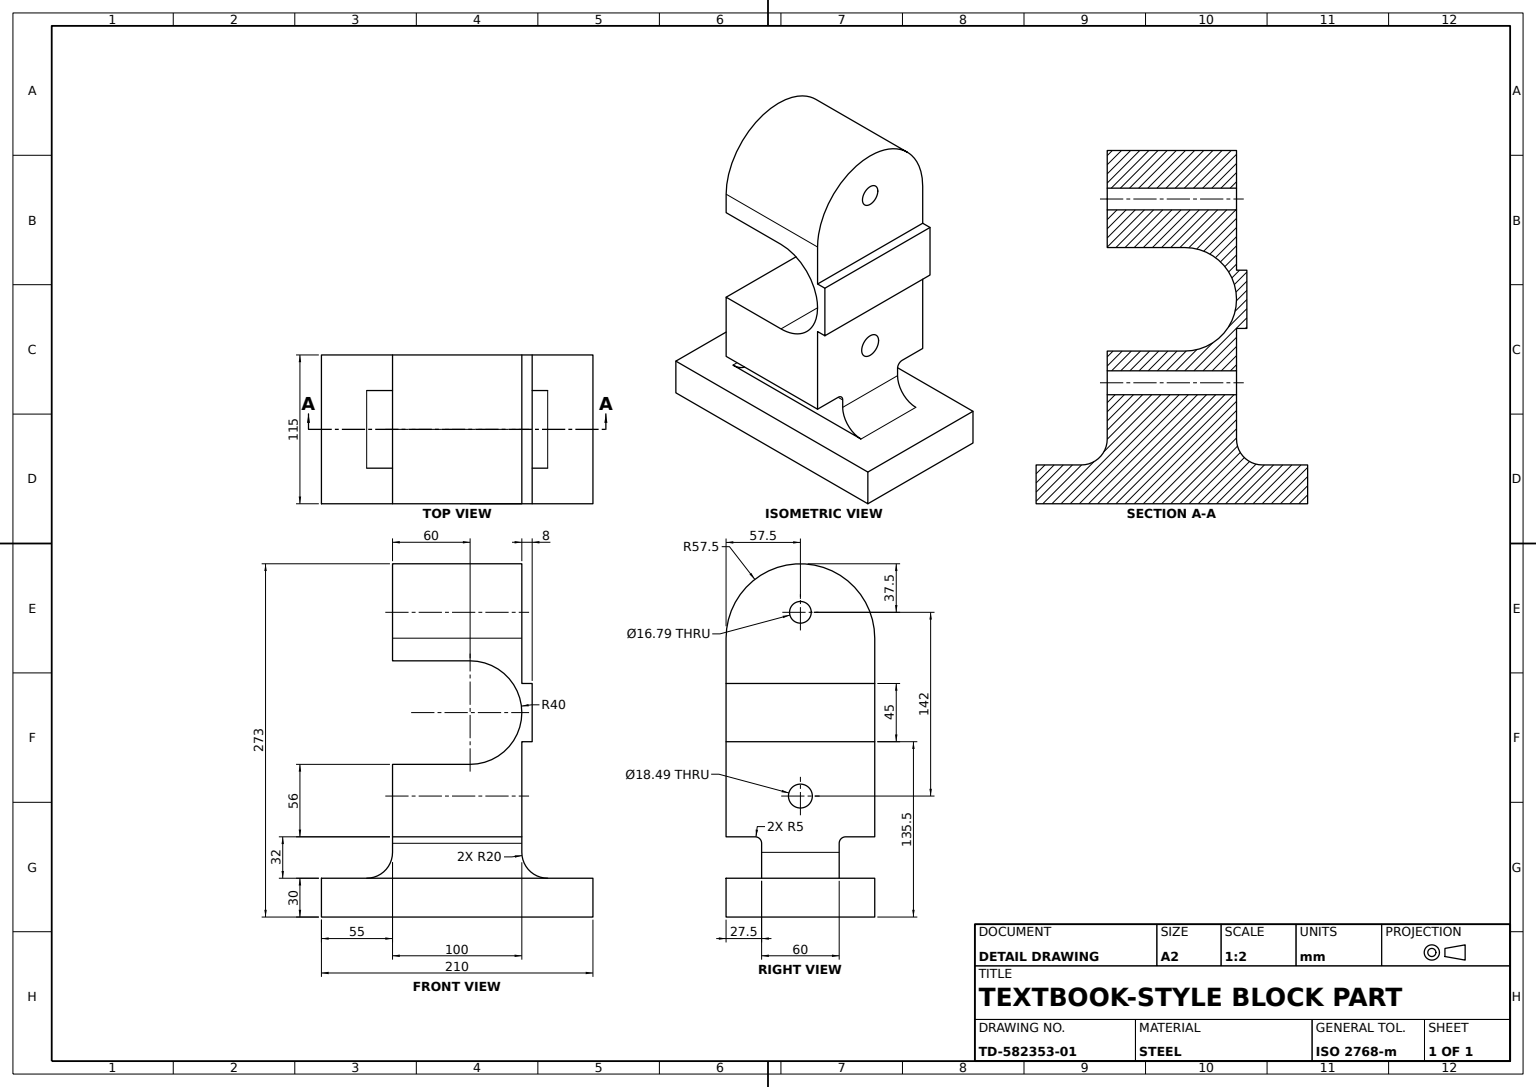
from build123d import *

# Parameters (mm, degrees)
BASE_PLATE_SKETCH_W         = 115
BASE_PLATE_SKETCH_H         = 210
BASE_PLATE_115X210X30_DEPTH = 15
UPRIGHT_PROFILE_SKETCH_R    = 8.394069109
UPRIGHT_PROFILE_SKETCH_R_2  = 9.244434853
UPRIGHT_BODY_DEPTH          = 50
UPRIGHT_ROUND_RADIUS        = 57.5
UPRIGHT_ROUND_LENGTH        = 100
SADDLE_CUT_DEPTH            = 75
SIDE_BOSS_SKETCH_W          = 8
SIDE_BOSS_SKETCH_H          = 45
SIDE_BOSS_DEPTH             = 57.5
EDGE_FILLET_R20_R           = 20


with BuildPart() as part:
    # Base Plate Sketch → Base Plate 115x210x30 (new, symmetric)
    with BuildSketch(Plane(origin=(0, 0, 0), x_dir=(1, 0, 0), z_dir=(0, 1, 0))):
        Rectangle(BASE_PLATE_SKETCH_W, BASE_PLATE_SKETCH_H)
    extrude(amount=BASE_PLATE_115X210X30_DEPTH, both=True)

    # Upright Profile Sketch → Upright Body (add, symmetric)
    with BuildSketch(Plane.XY):
        with BuildLine():
            Line((57.5, 47), (35, 47))
            ThreePointArc((35, 47), (31.464466094, 45.535533906), (30, 42))
            Line((30, 42), (30, 15))
            Line((30, 15), (-30, 15))
            Line((-30, 15), (-30, 42))
            ThreePointArc((-30, 42), (-31.464466094, 45.535533906), (-35, 47))
            Line((-35, 47), (-57.5, 47))
            Line((-57.5, 47), (-57.5, 258))
            Line((-57.5, 258), (57.5, 258))
            Line((57.5, 258), (57.5, 47))
        make_face()
        with Locations((0, 220.5)):
            Circle(UPRIGHT_PROFILE_SKETCH_R, mode=Mode.SUBTRACT)
        with Locations((0, 78.5)):
            Circle(UPRIGHT_PROFILE_SKETCH_R_2, mode=Mode.SUBTRACT)
    extrude(amount=UPRIGHT_BODY_DEPTH, both=True)

    # Upright Round: full round fillet: the end face becomes a half cylinder, R = half its width
    upright_round_face = Plane((0, 258, 0), x_dir=(0, 0, 1), z_dir=(0, 1, 0))  # on the end face: x along it, z out of the body
    upright_round_slab = upright_round_face.offset(-UPRIGHT_ROUND_RADIUS / 2) * Box(UPRIGHT_ROUND_LENGTH, 2 * UPRIGHT_ROUND_RADIUS, UPRIGHT_ROUND_RADIUS, mode=Mode.PRIVATE)  # the body's end, R deep
    upright_round_round = Plane((0, 200.5, 0), x_dir=(0, 1, 0), z_dir=(0, 0, 1)) * Cylinder(UPRIGHT_ROUND_RADIUS, UPRIGHT_ROUND_LENGTH, mode=Mode.PRIVATE)  # its axis R under the face
    add(upright_round_slab - upright_round_round, mode=Mode.SUBTRACT)

    # Saddle Cut Sketch → Saddle Cut (cut, symmetric)
    with BuildSketch(Plane(origin=(0, 0, 0), x_dir=(0, 0, -1), z_dir=(1, 0, 0))):
        with BuildLine():
            Line((-50, 183), (10, 183))
            ThreePointArc((10, 183), (50, 143), (10, 103))
            Line((10, 103), (-50, 103))
            Line((-50, 103), (-50, 183))
        make_face()
    extrude(amount=SADDLE_CUT_DEPTH, both=True, mode=Mode.SUBTRACT)


with BuildPart() as saddle_cut_piece_1:
    # of the separate pieces the step leaves, piece 1, a body of its own (saddle_cut_pieces)
    add(part.part.solids().sort_by_distance((-57.5, -15, -105))[0])



with BuildPart() as saddle_cut_piece_2:
    # of the separate pieces the step leaves, piece 2, a body of its own (saddle_cut_pieces)
    add(part.part.solids().sort_by_distance((-57.5, 200.5, -50))[0])


with BuildPart() as saddle_cut_piece_1_1:
    add(saddle_cut_piece_1.part)

    add(saddle_cut_piece_2.part)  # Side Boss merges Saddle Cut piece 2
    # Side Boss Sketch → Side Boss (add, symmetric)
    with BuildSketch(Plane(origin=(0, 0, 0), x_dir=(0, 0, -1), z_dir=(1, 0, 0))):
        with Locations((54, 143)):
            Rectangle(SIDE_BOSS_SKETCH_W, SIDE_BOSS_SKETCH_H)
    extrude(amount=SIDE_BOSS_DEPTH, both=True)

    # Edge Fillet R20
    edge_fillet_r20_edges = [saddle_cut_piece_1_1.edges().sort_by_distance(p)[0] for p in [
        (0, 15, 50),
        (0, 15, -50),
    ]]
    fillet(edge_fillet_r20_edges, radius=EDGE_FILLET_R20_R)


solid = saddle_cut_piece_1_1.part
